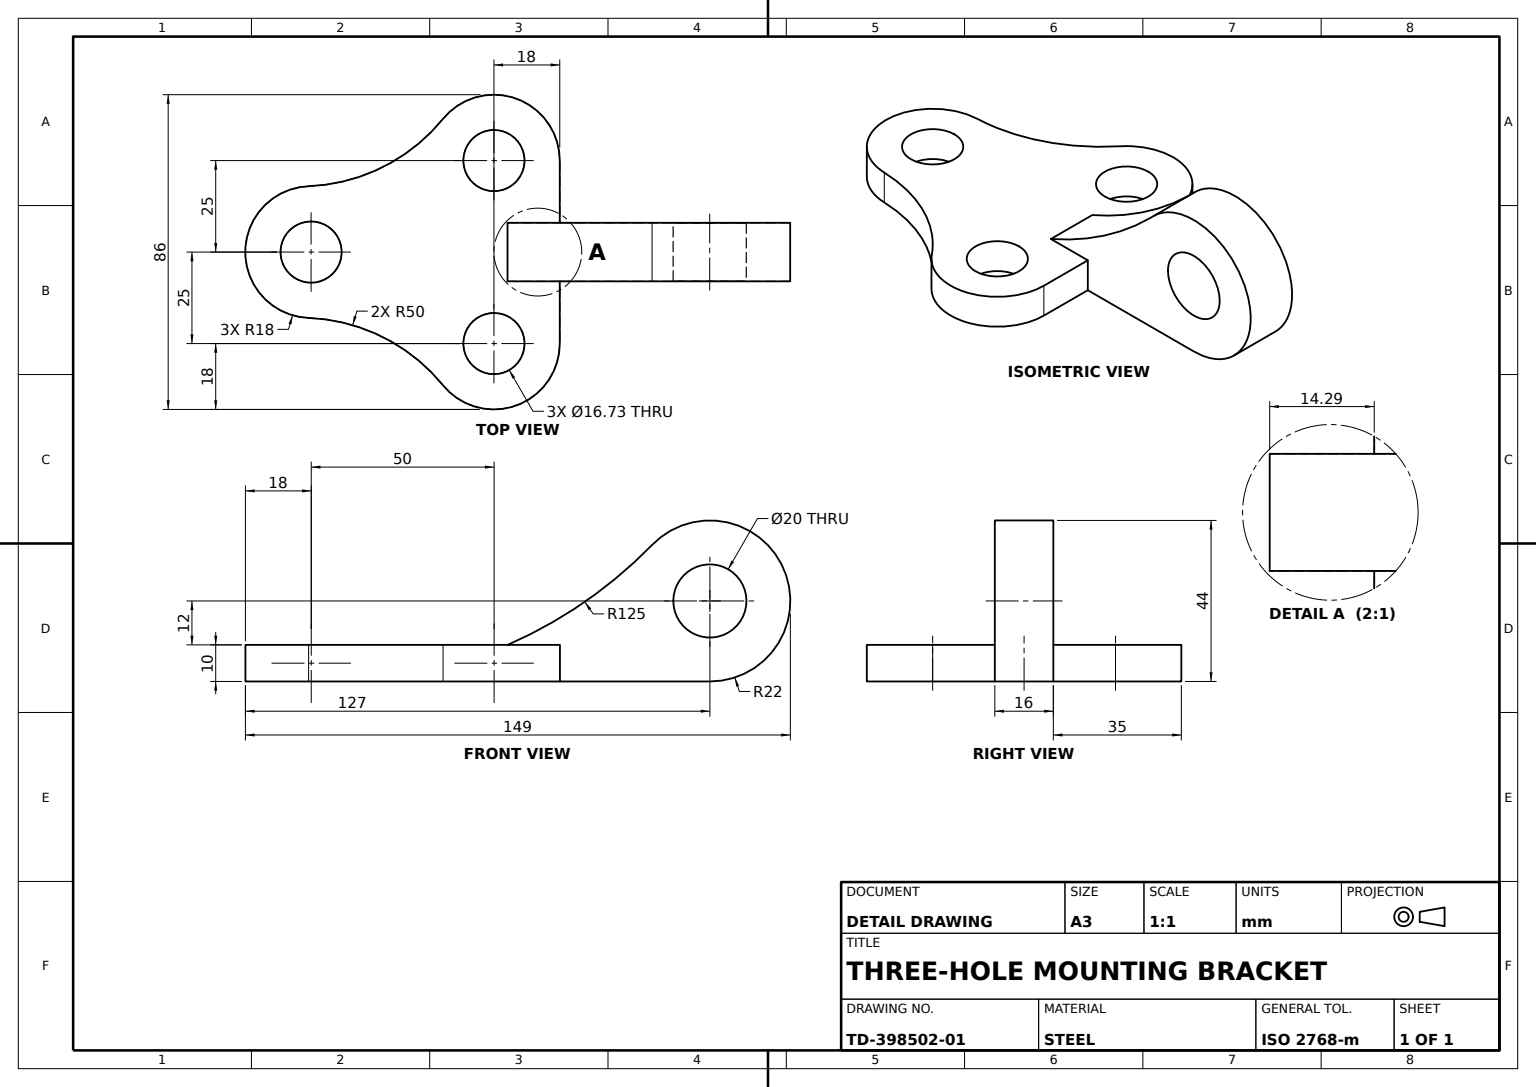
from build123d import *

# Parameters (mm, degrees)
BASE_PLATE_PROFILE_SKETCH_R = 8.363945013
BASE_PLATE_3_HOLE_DEPTH     = 10
BORED_LUG_PROFILE_SKETCH_R  = 10
BORED_LUG_DEPTH             = 8


with BuildPart() as part:
    # Base Plate Profile Sketch → Base Plate 3-Hole (new body)
    with BuildSketch(Plane(origin=(0, 0, 0), x_dir=(1, 0, 0), z_dir=(0, 1, 0))):
        with BuildLine():
            Line((68, 25), (68, -25))
            ThreePointArc((68, -25), (56.032896381, -41.958896227), (36.043982083, -36.367918187))
            ThreePointArc((36.043982083, -36.367918187), (19.637945422, -23.224109156), (-0.720723799, -17.985565246))
            ThreePointArc((-0.720723799, -17.985565246), (-18, 0), (-0.720723799, 17.985565246))
            ThreePointArc((-0.720723799, 17.985565246), (19.637945422, 23.224109156), (36.043982083, 36.367918187))
            ThreePointArc((36.043982083, 36.367918187), (56.032896381, 41.958896227), (68, 25))
        make_face()
        with Locations(Location((0, 0, 0), (0, 0, 270))):
            Circle(BASE_PLATE_PROFILE_SKETCH_R, mode=Mode.SUBTRACT)
        with Locations(Location((50, 25, 0), (0, 0, 270))):
            Circle(BASE_PLATE_PROFILE_SKETCH_R, mode=Mode.SUBTRACT)
        with Locations(Location((50, -25, 0), (0, 0, 90))):
            Circle(BASE_PLATE_PROFILE_SKETCH_R, mode=Mode.SUBTRACT)
    extrude(amount=BASE_PLATE_3_HOLE_DEPTH)

    # Bored Lug Profile Sketch → Bored Lug (add, symmetric)
    with BuildSketch(Plane.XY):
        with BuildLine():
            Line((68, 10), (53.71, 10))
            ThreePointArc((53.71, 10), (74.800840464, 21.756077977), (93.237910195, 37.347850827))
            ThreePointArc((93.237910195, 37.347850827), (129.268851943, 30.554159275), (109, 0))
            Line((109, 0), (68, 0))
            Line((68, 0), (68, 10))
        make_face()
        with Locations((109, 22)):
            Circle(BORED_LUG_PROFILE_SKETCH_R, mode=Mode.SUBTRACT)
    extrude(amount=BORED_LUG_DEPTH, both=True)


solid = part.part
